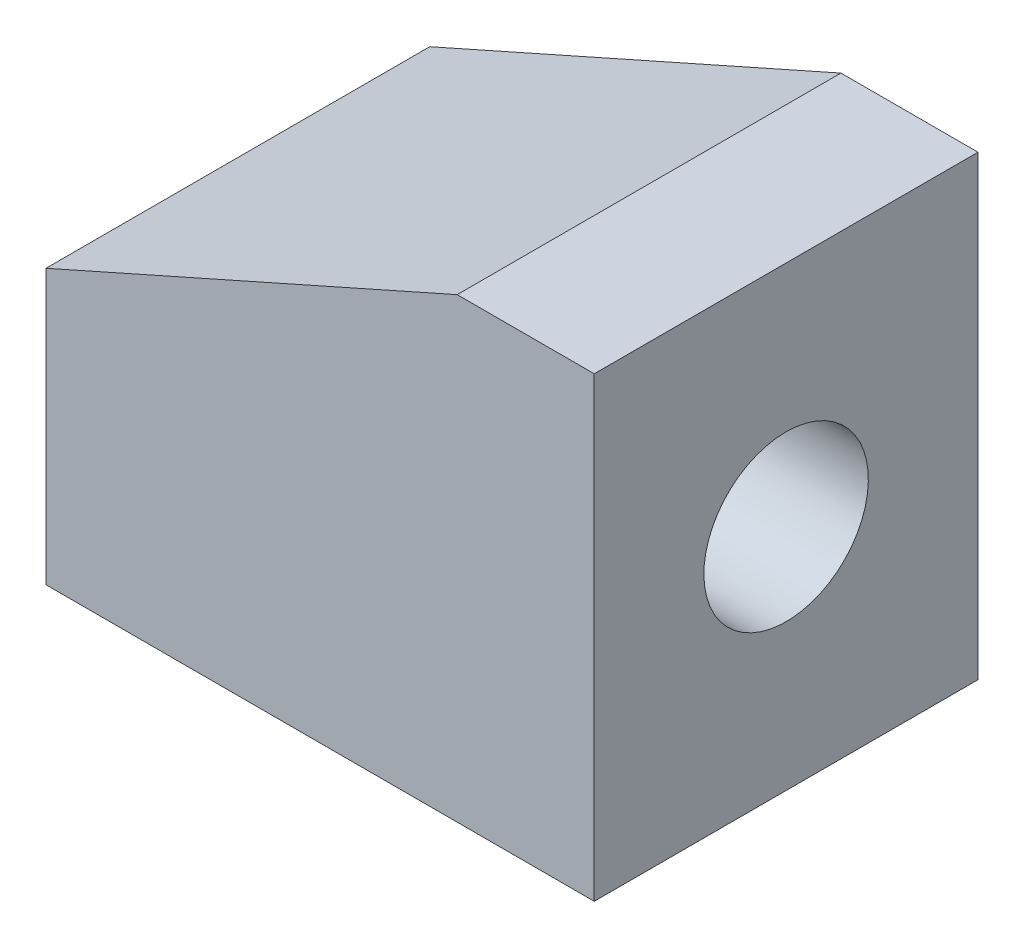
from build123d import *

# Parameters (mm, degrees)
BLOCK_BODY_DEPTH        = 21
BORE_18_SKETCH_R        = 9
BORE_18_X_40_DEEP_DEPTH = 40


with BuildPart() as part:
    # Block Profile Sketch → Block Body (new, symmetric)
    with BuildSketch(Plane.XY):
        Polygon((30, 0), (-30, 0), (-30, 30), (15, 50), (30, 50), align=None)
    extrude(amount=BLOCK_BODY_DEPTH, both=True)

    # Bore Ø18 Sketch → Bore Ø18 x 40 Deep (cut)
    with BuildSketch(Plane(origin=(30, 0, 0), x_dir=(0, 0, -1), z_dir=(1, 0, 0))):
        with Locations(Location((0, 25, 0), (0, 0, 90))):
            Circle(BORE_18_SKETCH_R)
    extrude(amount=-BORE_18_X_40_DEEP_DEPTH, mode=Mode.SUBTRACT)


solid = part.part
